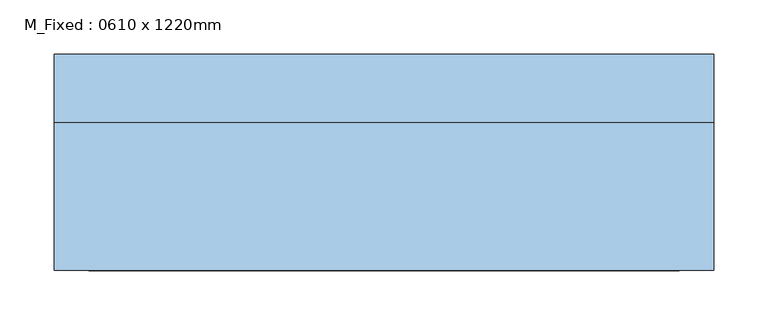
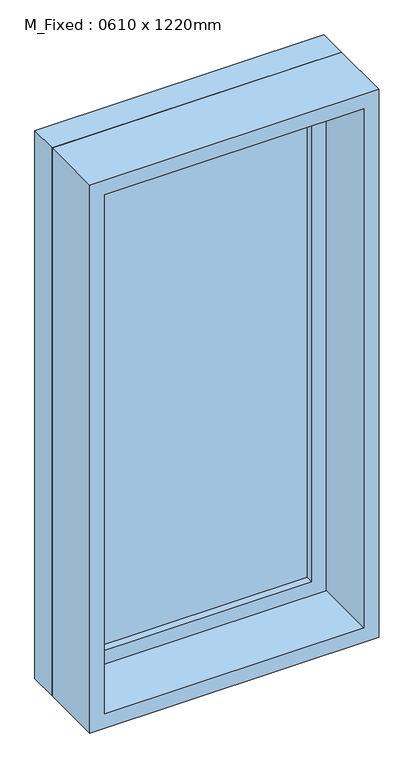
"""IFC4 building model written with IfcOpenShell, lengths in millimetres: window geometry, M_Fixed : 0610 x 1220mm."""

from ifc_helpers import new_model, si_unit, frame, origin, place, context, project, spatial, polyline, outline, extrude, source, transform, mapped, element, save


def m_fixed_0610_x_1220mm_4e981104(model_context):
    return source(origin(), model_context, "Body", "SweptSolid", [
        extrude(outline(polyline([(-242.0, 78.0), (242.0, 78.0), (242.0, 66.0), (-242.0, 66.0), (-242.0, 78.0)])), frame((0.0, 0.0, 978.0), z_axis=(0.0, 0.0, 1.0), x_axis=(1.0, 0.0, 0.0)), (0.0, 0.0, 1.0), 1094.0),
        extrude(outline(polyline([(2116.0, -286.0), (934.0, -286.0), (934.0, 286.0), (2116.0, 286.0), (2116.0, -286.0)]), holes=[polyline([(2072.0, -242.0), (2072.0, 242.0), (978.0, 242.0), (978.0, -242.0), (2072.0, -242.0)])]), frame((0.0, 50.0, 0.0), z_axis=(0.0, 1.0, 0.0), x_axis=(0.0, 0.0, 1.0)), (0.0, 0.0, 1.0), 44.0),
        extrude(outline(polyline([(2135.0, -305.0), (915.0, -305.0), (915.0, 305.0), (2135.0, 305.0), (2135.0, -305.0)]), holes=[polyline([(2116.0, -286.0), (2116.0, 286.0), (934.0, 286.0), (934.0, -286.0), (2116.0, -286.0)])]), frame((0.0, 50.0, 0.0), z_axis=(0.0, 1.0, 0.0), x_axis=(0.0, 0.0, 1.0)), (0.0, 0.0, 1.0), 63.0),
        extrude(outline(polyline([(2135.0, -305.0), (915.0, -305.0), (915.0, 305.0), (2135.0, 305.0), (2135.0, -305.0)]), holes=[polyline([(2103.0, -273.0), (2103.0, 273.0), (947.0, 273.0), (947.0, -273.0), (2103.0, -273.0)])]), frame((0.0, -87.0, 0.0), z_axis=(0.0, 1.0, 0.0), x_axis=(0.0, 0.0, 1.0)), (0.0, 0.0, 1.0), 137.0),
    ])


if __name__ == "__main__":
    model = new_model("IFC4")
    model_context = context("Model", 3, world=origin())
    ifc_project = project(units=[si_unit("LENGTHUNIT", "METRE", prefix="MILLI")], contexts=[model_context])
    site = spatial("IfcSite", under=ifc_project)
    building = spatial("IfcBuilding", under=site)
    placement = place(None, origin())
    m_fixed_0610_x_1220mm_shape = m_fixed_0610_x_1220mm_4e981104(model_context)
    element("IfcWindow", 1, ObjectType="M_Fixed : 0610 x 1220mm", at=placement, inside=building, context=model_context, shape_type="MappedRepresentation", body=[
        mapped(m_fixed_0610_x_1220mm_shape, transform((0.0, 0.0, 0.0), x_axis=(1.0, 0.0, 0.0), y_axis=(0.0, 1.0, 0.0), z_axis=(0.0, 0.0, 1.0))),
    ])
    save(model, "model.ifc")

# Revit data of these elements
# Type "M_Fixed : 0610 x 1220mm"
#   Type Mark = "13"
#   Height = 1220 mm
#   Default Sill Height = 915 mm
#   Width = 610 mm
#   Window Inset = 19 mm
#   Frame Exterior Material = Sash
#   Frame Interior Material = Sash
#   Glass Pane Material = Glass
#   Sash = Sash
#   Wall Closure = (empty or 0)
# Element 1 (IfcWindow, "M_Fixed : 0610 x 1220mm")
#   Materials on its faces: "Sash", "Glass"
# Materials
#   "Sash": class "Wood", colour RGB 136 99 55, transparency 0
#   "Glass": class "Glass", colour RGB 218 227 224, transparency 0.85, Description = "Soda Lime Glass", Cost = 0
